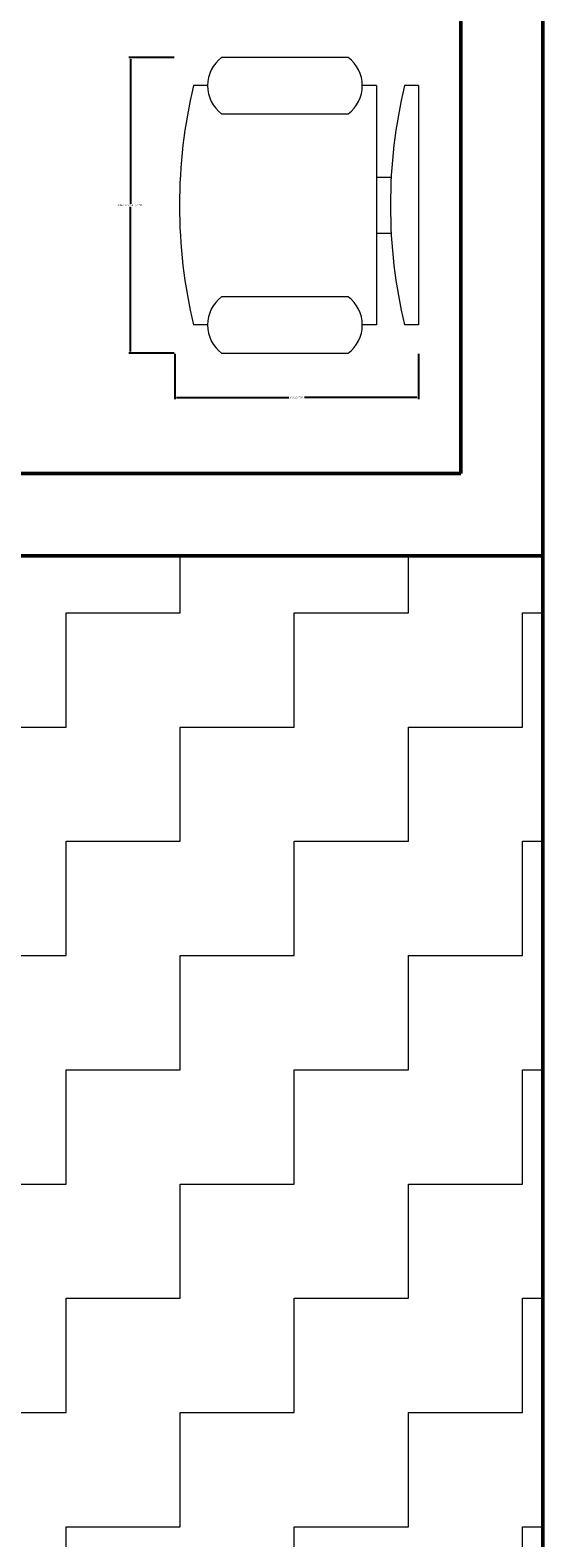
# Model space of a CAD drawing. Units: inches. Extents: x -105 to 1196, y -792 to 119.
# Tile 19 of 23: x 434 to 490, y -439 to -274. Entities that reach past the tile are written whole.
import ezdxf

# ---------------------------------------------------------------- set-up
doc = ezdxf.new("R2010")
doc.units = ezdxf.units.IN
doc.header["$MEASUREMENT"] = 0
for name, color, linetype, lineweight in [('A-ANNO-DIMS', 2, 'Continuous', 18), ('A-FLOR-PATT', 252, 'Continuous', 13), ('A-FURN', 8, 'Continuous', 18), ('A-WALL', 3, 'Continuous', 50)]:
    doc.layers.add(name, color=color, linetype=linetype, lineweight=lineweight)
doc.styles.get("Standard").update_dxf_attribs({"font": 'arial.ttf'})
doc.dimstyles.get("Standard").update_dxf_attribs({"dimtxt": 0.18, "dimasz": 0.18, "dimexe": 0.18, "dimexo": 0.0625, "dimgap": 0.09, "dimtad": 0, "dimtih": 1, "dimtoh": 1, "dimdec": 1, "dimzin": 0, "dimdsep": 46, "dimlunit": 4, "dimtxsty": 'Standard', "dimcen": 0.09, "dimadec": 0, "dimazin": 0, "dimtfac": 1, "dimtdec": 1, "dimtofl": 0, "dimtmove": 0, "dimatfit": 3, "dimfxl": 1, "dimtolj": 1, "dimtzin": 0, "dimarcsym": 0})

# ---------------------------------------------------------------- blocks, each defined once
blk = doc.blocks.new('Chair - Desk')
for p, q in [((-8.5, 0), (-8.5, -1)), ((-8.5, 0), (8.5, 0)), ((8.5, 0), (8.5, -1)), ((-2, -3), (-2, -1.9355)), ((2, -1.9576), (2, -3)), ((-8.5, -3), (-8.5, -4)), ((-8.5, -3), (8.5, -3)), ((8.5, -3), (8.5, -4)), ((-10.5, -5), (-10.5, -14)), ((-6.5, -14), (-6.5, -5)), ((6.5, -5), (6.5, -14)), ((10.5, -14), (10.5, -5)), ((-8.5, -15), (-8.5, -16)), ((8.5, -15), (8.5, -16))]:
    blk.add_line(p, q)
for centre, radius, start, end in [((0, 34.625), 36.625, 256.5803, 283.4197), ((-8.5, -6.5), 2.5, 36.8699, 143.1301), ((8.5, -6.5), 2.5, 36.8699, 143.1301), ((-8.5, -12.5), 2.5, 216.8699, 323.1301), ((8.5, -12.5), 2.5, 216.8699, 323.1301), ((0, 19.625), 36.625, 256.5803, 283.4197)]:
    blk.add_arc(centre, radius, start, end)
blk = doc.blocks.new('*D67')
at = {"layer": 'A-ANNO-DIMS', "color": 0, "lineweight": -2, "transparency": 16777216}
for p, q in [((449.36, -276.71), (444.39, -276.71)), ((444.57, -276.89), (444.57, -292.71)), ((444.57, -308.89), (444.57, -293.07)), ((449.36, -309.07), (444.39, -309.07))]:
    blk.add_line(p, q, dxfattribs=at)
at = {"layer": 'A-ANNO-DIMS', "color": 0, "transparency": 16777216}
for points in [[(444.54, -276.89), (444.6, -276.89), (444.57, -276.71)], [(444.54, -308.89), (444.6, -308.89), (444.57, -309.07)]]:
    blk.add_solid(points, dxfattribs=at)
at = {"layer": 'Defpoints', "color": 0, "transparency": 16777216}
for p in [(449.42, -276.71), (444.57, -309.07), (449.42, -309.07)]:
    blk.add_point(p, dxfattribs=at)
at = {"layer": 'A-ANNO-DIMS', "color": 0, "transparency": 16777216, "insert": (444.57, -292.89), "char_height": 0.18, "attachment_point": 5}
blk.add_mtext('\\A1;ARMCHAIR 2\'-8 1/2" TYP.', dxfattribs=at)
blk = doc.blocks.new('*D68')
at = {"layer": 'A-ANNO-DIMS', "color": 0, "lineweight": -2, "transparency": 16777216}
for p, q in [((449.42, -309.13), (449.42, -314.1)), ((476.13, -309.13), (476.13, -314.1)), ((449.6, -313.92), (461.92, -313.92)), ((475.95, -313.92), (463.62, -313.92))]:
    blk.add_line(p, q, dxfattribs=at)
at = {"layer": 'A-ANNO-DIMS', "color": 0, "transparency": 16777216}
for points in [[(449.6, -313.89), (449.6, -313.95), (449.42, -313.92)], [(475.95, -313.89), (475.95, -313.95), (476.13, -313.92)]]:
    blk.add_solid(points, dxfattribs=at)
at = {"layer": 'Defpoints', "color": 0, "transparency": 16777216}
for p in [(449.42, -309.07), (476.13, -309.07), (476.13, -313.92)]:
    blk.add_point(p, dxfattribs=at)
at = {"layer": 'A-ANNO-DIMS', "color": 0, "transparency": 16777216, "insert": (462.77, -313.92), "char_height": 0.18, "attachment_point": 5}
blk.add_mtext('\\A1;2\'-2 1/2" TYP.', dxfattribs=at)

msp = doc.modelspace()

# ---------------------------------------------------------------- hatches: boundary and pattern name
at = {"layer": 'A-FLOR-PATT'}
h = msp.add_hatch(dxfattribs=at)
h.set_pattern_fill('ZIGZAG', color=256, scale=100)
h.set_pattern_definition([(0, (0, 0), (12.5, 12.5), [12.5, -12.5]), (90, (12.5, 0), (-12.5, 12.5), [12.5, -12.5])])
h.paths.add_polyline_path([(489.74, -331.23), (323.74, -331.23), (323.74, -508.23), (489.74, -508.23)])
h.paths.add_polyline_path([(383.72, -476.81), (434.09, -476.81), (434.09, -454.42), (383.72, -454.42)], flags=24)

# ---------------------------------------------------------------- linework, layer by layer
at = {"layer": 'A-WALL'}
for p, q in [((480.74, -125.23), (480.74, -322.23)), ((489.74, -125.23), (489.74, -508.23)), ((480.74, -322.23), (323.74, -322.23)), ((489.74, -331.23), (323.74, -331.23))]:
    msp.add_line(p, q, dxfattribs=at)

# ---------------------------------------------------------------- block references
at = {"layer": 'A-FURN', "xscale": 1.540628433460857, "yscale": 1.540628433460857, "zscale": 1.540628433460857, "rotation": 270}
msp.add_blockref('Chair - Desk', (476.13, -292.89), dxfattribs=at)

# ---------------------------------------------------------------- dimensions: what is measured, and where the dimension line sits
at = {"layer": 'A-ANNO-DIMS'}
dim = msp.add_linear_dim(base=(444.57, -309.07), p1=(449.42, -276.71), p2=(449.42, -309.07), angle=270, text='ARMCHAIR <> TYP.', dimstyle='Standard', override={"dimdec": 1, "dimlfac": 1, "dimrnd": 0, "dimzin": 1, "dimdsep": 46, "dimlunit": 4, "dimfrac": 2}, dxfattribs=at)
dim.commit()
dim.dimension.update_dxf_attribs({"geometry": '*D67', "text_midpoint": (444.57, -292.89)})
dim = msp.add_linear_dim(base=(476.13, -313.92), p1=(449.42, -309.07), p2=(476.13, -309.07), text='<> TYP.', dimstyle='Standard', override={"dimdec": 1, "dimlfac": 1, "dimrnd": 0, "dimzin": 1, "dimdsep": 46, "dimlunit": 4, "dimfrac": 2}, dxfattribs=at)
dim.commit()
dim.dimension.update_dxf_attribs({"geometry": '*D68', "text_midpoint": (462.77, -313.92)})

doc.saveas('drawing.dxf')
